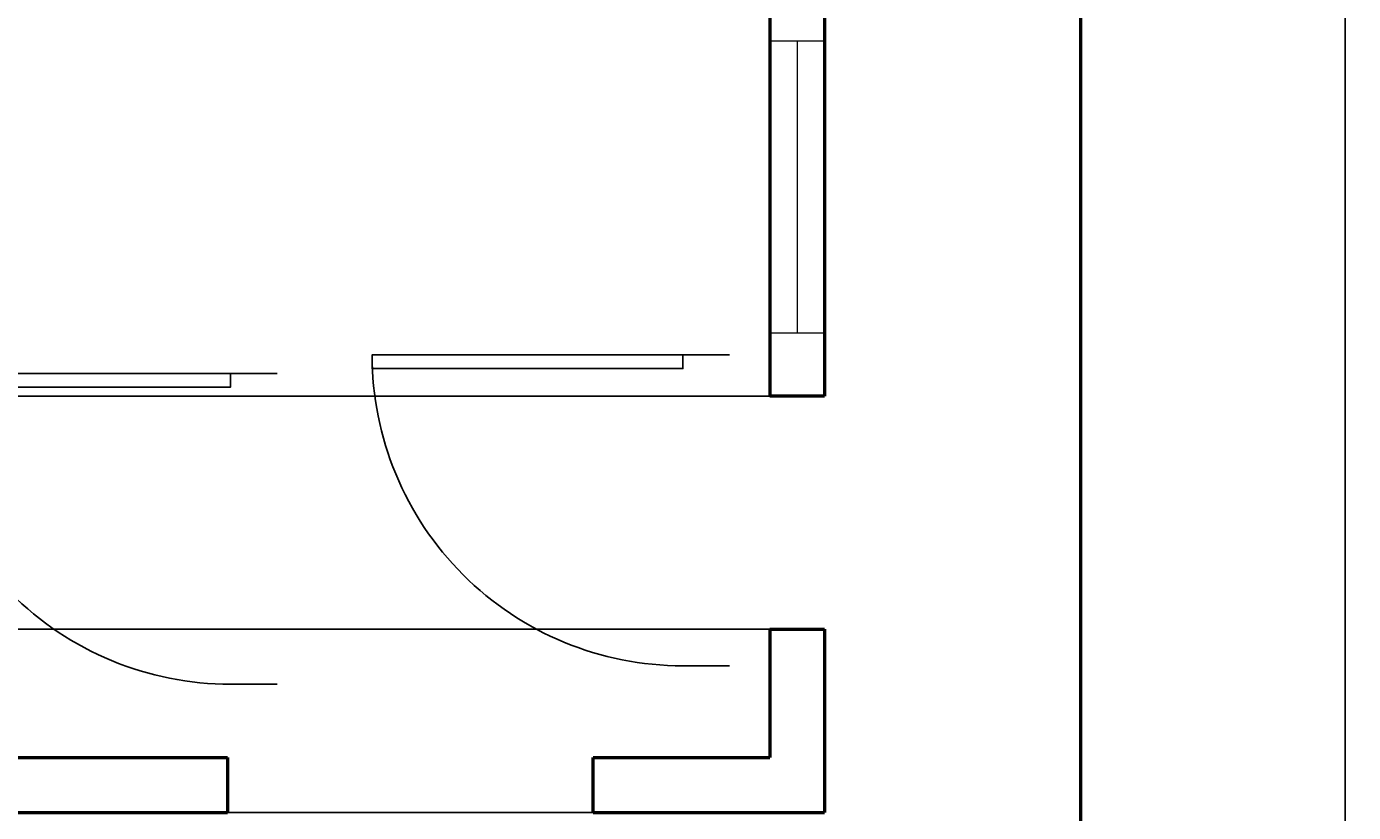
# Model space of a CAD drawing. Units: inches. Extents: x 3506 to 3958, y 1553 to 2506.
# Tile 7 of 16: x 3739 to 3957, y 1770 to 1899. Entities that reach past the tile are written whole.
import ezdxf

# ---------------------------------------------------------------- set-up
doc = ezdxf.new("R2010")
doc.units = ezdxf.units.IN
doc.header["$MEASUREMENT"] = 0
for name, color, linetype, lineweight in [('A-ANNO-DIMS', 2, 'Continuous', 18), ('A-FLOR-STRS', 7, 'Continuous', 25), ('A-WALL', 7, 'Continuous', 50), ('doors', 40, 'Continuous', 25), ('window', 30, 'Continuous', 20)]:
    doc.layers.add(name, color=color, linetype=linetype, lineweight=lineweight)
doc.layers.add('A-WALL-PATT', color=251, linetype='Continuous', lineweight=13, true_color=0x636466)
doc.styles.get("Standard").update_dxf_attribs({"font": 'arial.ttf'})
doc.dimstyles.get("Standard").update_dxf_attribs({"dimtxt": 1.18, "dimasz": 0.68, "dimexe": 0.18, "dimexo": 0.0625, "dimgap": 0.09, "dimtad": 0, "dimtih": 1, "dimtoh": 1, "dimdec": 1, "dimzin": 0, "dimdsep": 46, "dimlunit": 3, "dimtxsty": 'Standard', "dimcen": 0.09, "dimadec": 0, "dimazin": 0, "dimtfac": 1, "dimtdec": 1, "dimtofl": 0, "dimtmove": 0, "dimatfit": 3, "dimfxl": 1, "dimtolj": 1, "dimtzin": 0, "dimarcsym": 0})

# ---------------------------------------------------------------- blocks, each defined once
blk = doc.blocks.new('*U12')
for p, q in [((0, 0), (0, 6)), ((40, 0), (40, 6))]:
    blk.add_line(p, q)
blk.add_lwpolyline([(0, 0), (0, -40), (1.75, -40), (1.75, 0)], close=True)
blk.add_arc((0, 0), 40, 270, 0)
blk = doc.blocks.new('*D39')
at = {"layer": 'A-ANNO-DIMS', "color": 0, "lineweight": -2, "transparency": 16777216}
for p, q in [((3911.79, 2461.39), (3955.36, 2461.39)), ((3955.18, 2460.71), (3955.18, 2030.09)), ((3955.18, 1598.07), (3955.18, 2028.7)), ((3911.79, 1597.39), (3955.36, 1597.39))]:
    blk.add_line(p, q, dxfattribs=at)
at = {"layer": 'A-ANNO-DIMS', "color": 0, "transparency": 16777216}
for points in [[(3955.07, 2460.71), (3955.29, 2460.71), (3955.18, 2461.39)], [(3955.07, 1598.07), (3955.29, 1598.07), (3955.18, 1597.39)]]:
    blk.add_solid(points, dxfattribs=at)
at = {"layer": 'Defpoints', "color": 0, "transparency": 16777216}
for p in [(3911.73, 2461.39), (3955.18, 2461.39), (3911.73, 1597.39)]:
    blk.add_point(p, dxfattribs=at)
at = {"layer": 'A-ANNO-DIMS', "color": 0, "transparency": 16777216, "insert": (3955.18, 2029.39), "char_height": 1.18, "attachment_point": 5}
blk.add_mtext('\\A1;864', dxfattribs=at)
blk = doc.blocks.new('*D62')
at = {"layer": 'A-ANNO-DIMS', "color": 0, "lineweight": -2, "transparency": 16777216}
for p, q in [((3860.67, 1838.71), (3508.1, 1838.71)), ((3508.28, 1838.03), (3508.28, 1820.28)), ((3508.28, 1801.14), (3508.28, 1818.89)), ((3860.67, 1800.46), (3508.1, 1800.46))]:
    blk.add_line(p, q, dxfattribs=at)
at = {"layer": 'A-ANNO-DIMS', "color": 0, "transparency": 16777216}
for points in [[(3508.17, 1838.03), (3508.39, 1838.03), (3508.28, 1838.71)], [(3508.17, 1801.14), (3508.39, 1801.14), (3508.28, 1800.46)]]:
    blk.add_solid(points, dxfattribs=at)
at = {"layer": 'Defpoints', "color": 0, "transparency": 16777216}
for p in [(3860.73, 1838.71), (3508.28, 1800.46), (3860.73, 1800.46)]:
    blk.add_point(p, dxfattribs=at)
at = {"layer": 'A-ANNO-DIMS', "color": 0, "transparency": 16777216, "insert": (3508.28, 1819.59), "char_height": 1.18, "attachment_point": 5}
blk.add_mtext('\\A1;38.246', dxfattribs=at)
blk = doc.blocks.new('*D63')
at = {"layer": 'A-ANNO-DIMS', "color": 0, "lineweight": -2, "transparency": 16777216}
for p, q in [((3869.67, 1800.46), (3508.1, 1800.46)), ((3508.28, 1799.78), (3508.28, 1786.12)), ((3508.28, 1771.07), (3508.28, 1784.74)), ((3869.67, 1770.39), (3508.1, 1770.39))]:
    blk.add_line(p, q, dxfattribs=at)
at = {"layer": 'A-ANNO-DIMS', "color": 0, "transparency": 16777216}
for points in [[(3508.17, 1799.78), (3508.39, 1799.78), (3508.28, 1800.46)], [(3508.17, 1771.07), (3508.39, 1771.07), (3508.28, 1770.39)]]:
    blk.add_solid(points, dxfattribs=at)
at = {"layer": 'Defpoints', "color": 0, "transparency": 16777216}
for p in [(3869.73, 1800.46), (3508.28, 1770.39), (3869.73, 1770.39)]:
    blk.add_point(p, dxfattribs=at)
at = {"layer": 'A-ANNO-DIMS', "color": 0, "transparency": 16777216, "insert": (3508.28, 1785.43), "char_height": 1.18, "attachment_point": 5}
blk.add_mtext('\\A1;30.07', dxfattribs=at)

msp = doc.modelspace()

# ---------------------------------------------------------------- hatches: boundary and pattern name
at = {"layer": 'A-WALL-PATT'}
h = msp.add_hatch(dxfattribs=at)
h.set_pattern_fill('ANSI31', color=256)
h.paths.add_polyline_path([(3911.7302, 2461.3942), (3551.7302, 2461.3942), (3551.7302, 2152.516), (3560.7302, 2152.516), (3560.7302, 2116.516), (3551.7302, 2116.516), (3551.7302, 1920.5711), (3556.2302, 1920.5711), (3560.7302, 1920.5711), (3560.7302, 2000.3942), (3692.7302, 2000.3942), (3692.7302, 1997.3942), (3697.7302, 1997.3942), (3697.7302, 2000.3942), (3771.7302, 2000.3942), (3771.7302, 1997.3942), (3776.7302, 1997.3942), (3776.7302, 1997.7206), (3778.5802, 1997.7206), (3807.5802, 1997.7206), (3807.5802, 1996.4519), (3778.5802, 1996.4519), (3778.5802, 1997.7206), (3776.7302, 1997.7206), (3776.7302, 1997.3942), (3771.7302, 1997.3942), (3771.7302, 2000.3942), (3697.7302, 2000.3942), (3697.7302, 1997.3942), (3692.7302, 1997.3942), (3689.8302, 1997.3942), (3689.8302, 1995.8192), (3653.8302, 1995.8192), (3653.8302, 1997.3942), (3689.8302, 1997.3942), (3692.7302, 1997.3942), (3692.7302, 2000.3942), (3560.7302, 2000.3942), (3560.7302, 1920.5711), (3551.7302, 1920.5711), (3551.7302, 1884.5711), (3551.7302, 1597.3942), (3911.7302, 1597.3942)], flags=17)
h.paths.add_polyline_path([(3596.7302, 2005.3942), (3596.7302, 2057.3035, -0.38730371), (3569.1778, 2085), (3569.15, 2085), (3569.15, 2086.2688), (3598.15, 2086.2688), (3598.15, 2085), (3569.1778, 2085, 0.38730371), (3596.7302, 2057.3035), (3596.7302, 2057.3942), (3601.7302, 2057.3942), (3601.7302, 2055.3942), (3630.7302, 2055.3942), (3630.7302, 2034.3942), (3694.7302, 2034.3942), (3694.7302, 2053.3942), (3699.7302, 2053.3942), (3699.7302, 2005.3942), (3860.7302, 2005.3942), (3860.7302, 2173.3942), (3771.7302, 2173.3942), (3771.7302, 2194.3942), (3776.7302, 2194.3942), (3776.7302, 2178.3942), (3860.7302, 2178.3942), (3860.7302, 2231.3942), (3601.7302, 2231.3942), (3601.7302, 2241.426), (3596.7302, 2241.426), (3596.7302, 2231.3942), (3560.7302, 2231.3942), (3560.7302, 2315.3942), (3596.7302, 2315.3942), (3596.7302, 2312.3942), (3601.7302, 2312.3942), (3601.7302, 2315.3942), (3697.7302, 2315.3942), (3697.7302, 2413.3942), (3692.7302, 2413.3942), (3692.7302, 2320.3942), (3560.7302, 2320.3942), (3560.7302, 2452.3942), (3692.7302, 2452.3942), (3692.7302, 2449.3942), (3697.7302, 2449.3942), (3697.7302, 2452.3942), (3771.7302, 2452.3942), (3771.7302, 2449.3942), (3776.7302, 2449.3942), (3776.7302, 2452.3942), (3860.7302, 2452.3942), (3860.7302, 2437.2075), (3865.2302, 2437.2075), (3865.2302, 2413.2075), (3860.7302, 2413.2075), (3860.7302, 2367.6976), (3865.2302, 2367.6976), (3869.7302, 2367.6976), (3869.7302, 2319.6976), (3860.7302, 2319.6976), (3860.7302, 2211.6248), (3869.7302, 2211.6248), (3869.7302, 2187.6248), (3860.7302, 2187.6248), (3860.7302, 2138.4346), (3865.2302, 2138.4346), (3869.7302, 2138.4346), (3869.7302, 2090.4346), (3860.7302, 2090.4346), (3860.7302, 1985.8449), (3869.7302, 1985.8449), (3869.7302, 1961.8449), (3860.7302, 1961.8449), (3860.7302, 1897.0756), (3865.2302, 1897.0756), (3869.7302, 1897.0756), (3869.7302, 1849.0756), (3860.7302, 1849.0756), (3860.7302, 1847.8112), (3860.7302, 1779.3942), (3596.7302, 1779.3942), (3596.7302, 1831.3942), (3601.7302, 1831.3942), (3601.7302, 1828.3942), (3630.7302, 1828.3942), (3630.7302, 1808.3942), (3691.7302, 1808.3942), (3691.7302, 1815.3942), (3696.7302, 1815.3942), (3696.7302, 1779.3942), (3860.7302, 1779.3942), (3860.7302, 1947.3942), (3771.7302, 1947.3942), (3771.7302, 1968.3942), (3776.7302, 1968.3942), (3776.7302, 1952.3942), (3860.7302, 1952.3942), (3860.7302, 2005.3942)], flags=0)
h.paths.add_polyline_path([(3596.7302, 2038.8546), (3601.7302, 2038.8546), (3601.7302, 2014.8546), (3596.7302, 2014.8546)], flags=0)
h.paths.add_polyline_path([(3564.1688, 2107), (3564.1688, 2167), (3644.1688, 2167), (3644.1688, 2107)], flags=0)
h.paths.add_polyline_path([(3607.0972, 2052.0208), (3620.8472, 2052.0208, -0.41421356), (3621.9931, 2050.875), (3621.9931, 2025.6667, -0.41421356), (3620.8472, 2024.5208), (3607.0972, 2024.5208, -0.41421356), (3605.9514, 2025.6667), (3605.9514, 2050.875, -0.41421356)], flags=0)
h.paths.add_polyline_path([(3578.5688, 2115), (3565.3688, 2115), (3565.3688, 2135.8), (3578.5688, 2135.8), (3578.5688, 2138.2), (3565.3688, 2138.2), (3565.3688, 2159), (3580.5688, 2159), (3580.5688, 2153.8), (3593.7688, 2167), (3593.7688, 2151.8), (3578.5688, 2151.8)], flags=0)
h.paths.add_polyline_path([(3610.9167, 2050.875), (3620.0833, 2050.875, -0.41421356), (3620.8472, 2050.1111), (3620.8472, 2039.6076, -0.41421356), (3620.0833, 2038.8438), (3610.9167, 2038.8438, -0.41421356), (3610.1528, 2039.6076), (3610.1528, 2050.1111, -0.41421356)], flags=0)
h.paths.add_polyline_path([(3610.9167, 2037.6979), (3620.0833, 2037.6979, -0.41421356), (3620.8472, 2036.934), (3620.8472, 2026.4306, -0.41421356), (3620.0833, 2025.6667), (3610.9167, 2025.6667, -0.41421356), (3610.1528, 2026.4306), (3610.1528, 2036.934, -0.41421356)], flags=0)
h.paths.add_polyline_path([(3616.2639, 2044.7639, -1), (3614.7361, 2044.7639, -1)], flags=0)
h.paths.add_polyline_path([(3615.8819, 2044.7639, -1), (3615.1181, 2044.7639, -1)], flags=0)
h.paths.add_polyline_path([(3616.2639, 2031.7778, -1), (3614.7361, 2031.7778, -1)], flags=0)
h.paths.add_polyline_path([(3615.8819, 2031.7778, -1), (3615.1181, 2031.7778, -1)], flags=0)
h.paths.add_polyline_path([(3609.7539, 2021.7868), (3626.9586, 2021.7868), (3626.9586, 2008.8833), (3609.7539, 2008.8833)], flags=0)
h.paths.add_polyline_path([(3610.4708, 2021.07), (3621.2237, 2021.07), (3621.2237, 2009.6002), (3610.4708, 2009.6002)], flags=0)
h.paths.add_polyline_path([(3611.5461, 2019.9947), (3620.1484, 2019.9947), (3620.1484, 2010.6755), (3611.5461, 2010.6755)], flags=0)
h.paths.add_polyline_path([(3621.9405, 2021.07), (3626.2417, 2021.07), (3626.2417, 2009.6002), (3621.9405, 2009.6002)], flags=0)
h.paths.add_polyline_path([(3622.6574, 2020.3531), (3625.5248, 2020.3531), (3625.5248, 2017.4857), (3622.6574, 2017.4857)], flags=0)
h.paths.add_polyline_path([(3622.6574, 2016.7688), (3625.5248, 2016.7688), (3625.5248, 2010.317), (3622.6574, 2010.317)], flags=0)
h.paths.add_polyline_path([(3624.808, 2016.0519), (3624.808, 2013.9013), (3624.0911, 2013.9013), (3624.0911, 2013.1845), (3623.3743, 2013.1845), (3623.3743, 2013.9013), (3623.3743, 2016.0519)], flags=0)
h.paths.add_polyline_path([(3623.0158, 2012.8261), (3625.1664, 2012.8261), (3625.1664, 2012.1092), (3623.0158, 2012.1092)], flags=0)
h.paths.add_polyline_path([(3623.0158, 2011.7508), (3625.1664, 2011.7508), (3625.1664, 2011.0339), (3623.0158, 2011.0339)], flags=0)
h.paths.add_polyline_path([(3650.0591, 2031.8202), (3674.0368, 2031.8202), (3674.0368, 2012.638), (3669.2413, 2012.638), (3669.2413, 2011.8388), (3672.4383, 2011.8388), (3672.4383, 2011.0395), (3651.6576, 2011.0395), (3651.6576, 2011.8388), (3654.8546, 2011.8388), (3654.8546, 2012.638), (3650.0591, 2012.638)], flags=0)
h.paths.add_polyline_path([(3658.0517, 2024.6269, -1), (3651.6576, 2024.6269, -1)], flags=0)
h.paths.add_polyline_path([(3657.2524, 2024.6269, -1), (3652.4569, 2024.6269, -1)], flags=0)
h.paths.add_polyline_path([(3656.4532, 2024.6269, -1), (3653.2561, 2024.6269, -1)], flags=0)
h.paths.add_polyline_path([(3655.6539, 2024.6269, -1), (3654.0554, 2024.6269, -1)], flags=0)
h.paths.add_polyline_path([(3657.2524, 2017.4336, -1), (3652.4569, 2017.4336, -1)], flags=0)
h.paths.add_polyline_path([(3656.4532, 2017.4336, -1), (3653.2561, 2017.4336, -1)], flags=0)
h.paths.add_polyline_path([(3655.6539, 2017.4336, -1), (3654.0554, 2017.4336, -1)], flags=0)
h.paths.add_polyline_path([(3659.6502, 2027.8239), (3664.4457, 2027.8239), (3664.4457, 2015.0358), (3659.6502, 2015.0358)], flags=0)
h.paths.add_polyline_path([(3663.6465, 2027.0247), (3663.6465, 2015.8351), (3660.4494, 2015.8351), (3660.4494, 2027.0247)], flags=0)
h.paths.add_polyline_path([(3562.6688, 1945.5), (3642.6688, 1945.5), (3642.6688, 1885.5), (3562.6688, 1885.5)], flags=0)
h.paths.add_polyline_path([(3671.6391, 2024.6269, -1), (3666.8435, 2024.6269, -1)], flags=0)
h.paths.add_polyline_path([(3670.8398, 2024.6269, -1), (3667.6428, 2024.6269, -1)], flags=0)
h.paths.add_polyline_path([(3672.4383, 2017.4336, -1), (3666.0443, 2017.4336, -1)], flags=0)
h.paths.add_polyline_path([(3670.0405, 2024.6269, -1), (3668.442, 2024.6269, -1)], flags=0)
h.paths.add_polyline_path([(3671.6391, 2017.4336, -1), (3666.8435, 2017.4336, -1)], flags=0)
h.paths.add_polyline_path([(3670.8398, 2017.4336, -1), (3667.6428, 2017.4336, -1)], flags=0)
h.paths.add_polyline_path([(3592.2688, 1945.5), (3592.2688, 1930.3), (3577.0688, 1930.3), (3577.0688, 1893.5), (3563.8688, 1893.5), (3563.8688, 1914.3), (3577.0688, 1914.3), (3577.0688, 1916.7), (3563.8688, 1916.7), (3563.8688, 1937.5), (3579.0688, 1937.5), (3579.0688, 1932.3)], flags=0)
h.paths.add_polyline_path([(3670.0405, 2017.4336, -1), (3668.442, 2017.4336, -1)], flags=0)
h.paths.add_polyline_path([(3596.7302, 2283.3942), (3601.7302, 2283.3942), (3601.7302, 2265.426), (3599.2302, 2265.426), (3599.2302, 2241.426), (3596.7302, 2241.426), (3596.7302, 2265.426)], flags=0)
h.paths.add_polyline_path([(3596.7302, 1810.7006), (3601.7302, 1810.7006), (3601.7302, 1786.7006), (3596.7302, 1786.7006)], flags=0)
h.paths.add_polyline_path([(3560.7302, 1770.3942), (3738.7302, 1770.3942), (3738.7302, 1746.3942), (3738.7302, 1722.3942), (3748.7302, 1722.3942), (3748.7302, 1674.3942), (3560.7302, 1674.3942)], flags=0)
h.paths.add_polyline_path([(3728.7302, 1746.3942), (3728.7302, 1756.0642), (3738.7302, 1746.3942), (3728.7302, 1738.1582), (3728.7302, 1698.3942), (3591.2519, 1698.3942), (3591.2519, 1746.3942)], flags=0)
h.paths.add_polyline_path([(3771.7302, 2399.3942), (3771.7302, 2420.3942), (3776.7302, 2420.3942), (3776.7302, 2404.3942), (3776.7302, 2399.3942)], flags=0)
h.paths.add_polyline_path([(3911.7302, 2461.3942), (3551.7302, 2461.3942), (3551.7302, 2152.516), (3560.7302, 2152.516), (3560.7302, 2116.516), (3551.7302, 2116.516), (3551.7302, 1920.5711), (3560.7302, 1920.5711), (3560.7302, 2000.3942), (3692.7302, 2000.3942), (3692.7302, 1997.3942), (3697.7302, 1997.3942), (3697.7302, 2000.3942), (3771.7302, 2000.3942), (3771.7302, 1997.3942), (3776.7302, 1997.3942), (3776.7302, 1997.7206), (3778.5802, 1997.7206), (3807.5802, 1997.7206), (3807.5802, 1996.4519), (3778.5802, 1996.4519), (3778.5802, 1997.7206), (3776.7302, 1997.7206), (3776.7302, 1997.3942), (3771.7302, 1997.3942), (3771.7302, 2000.3942), (3697.7302, 2000.3942), (3697.7302, 1997.3942), (3692.7302, 1997.3942), (3689.8302, 1997.3942), (3689.8302, 1995.8192), (3653.8302, 1995.8192), (3653.8302, 1997.3942), (3689.8302, 1997.3942), (3692.7302, 1997.3942), (3692.7302, 2000.3942), (3560.7302, 2000.3942), (3560.7302, 1920.5711), (3551.7302, 1920.5711), (3551.7302, 1597.3942), (3911.7302, 1597.3942)], flags=17)

# ---------------------------------------------------------------- linework, layer by layer
at = {"layer": 'A-FLOR-STRS'}
msp.add_line((3608.7302, 1770.3942), (3771.7302, 1770.3942), dxfattribs=at)
at = {"layer": 'A-WALL'}
for p, q in [((3860.7302, 2015.4906), (3860.7302, 1838.7087)), ((3869.7302, 2015.4906), (3869.7302, 1838.7087)), ((3869.7302, 1838.7087), (3860.7302, 1838.7087)), ((3860.7302, 1800.4628), (3869.7302, 1800.4628)), ((3860.7302, 1800.4628), (3860.7302, 1779.3942)), ((3869.7302, 1800.4628), (3869.7302, 1770.3942)), ((3560.7302, 1779.3942), (3771.7302, 1779.3942)), ((3771.7302, 1779.3942), (3771.7302, 1770.3942)), ((3831.7302, 1779.3942), (3860.7302, 1779.3942)), ((3831.7302, 1770.3942), (3831.7302, 1779.3942)), ((3831.7302, 1779.3942), (3860.7302, 1779.3942)), ((3560.7302, 1770.3942), (3771.7302, 1770.3942)), ((3831.7302, 1770.3942), (3860.7302, 1770.3942)), ((3831.7302, 1770.3942), (3869.7302, 1770.3942))]:
    msp.add_line(p, q, dxfattribs=at)
msp.add_lwpolyline([(3551.7302, 2461.3942), (3911.7302, 2461.3942), (3911.7302, 1597.3942), (3551.7302, 1597.3942)], close=True, dxfattribs=at)
at = {"layer": 'window'}
for p, q in [((3860.7302, 1897.0756), (3869.7302, 1897.0756)), ((3860.7302, 1897.0756), (3865.2302, 1897.0756)), ((3865.2302, 1897.0756), (3865.2302, 1849.0756)), ((3869.7302, 1897.0756), (3869.7302, 1849.0756)), ((3860.7302, 1895.8112), (3860.7302, 1847.8112)), ((3869.7302, 1849.0756), (3860.7302, 1849.0756))]:
    msp.add_line(p, q, dxfattribs=at)

# ---------------------------------------------------------------- block references
at = {"layer": 'doors', "xscale": 1.27563568336709, "yscale": 1.27563568336709, "zscale": 1.27563568336709, "rotation": 270}
for p in [(3846.4757, 1845.4859), (3772.2282, 1842.4626)]:
    msp.add_blockref('*U12', p, dxfattribs=at)

# ---------------------------------------------------------------- dimensions: what is measured, and where the dimension line sits
at = {"layer": 'A-ANNO-DIMS'}
for base, p1, p2, override, picture, middle in [((3955.1802, 2461.3942), (3911.7302, 1597.3942), (3911.7302, 2461.3942), {"dimdec": 0, "dimlfac": 1, "dimrnd": 0, "dimzin": 0, "dimdsep": 46, "dimlunit": 2}, '*D39', (3955.1802, 2029.3942)), ((3508.2802, 1800.4628), (3860.7302, 1838.7087), (3860.7302, 1800.4628), {"dimdec": 3, "dimlfac": 1, "dimrnd": 0, "dimzin": 0, "dimdsep": 46, "dimlunit": 2}, '*D62', (3508.2802, 1819.5857)), ((3508.2802, 1770.3942), (3869.7302, 1800.4628), (3869.7302, 1770.3942), {"dimdec": 2, "dimlfac": 1, "dimrnd": 0, "dimzin": 0, "dimdsep": 46, "dimlunit": 2}, '*D63', (3508.2802, 1785.4285))]:
    dim = msp.add_linear_dim(base=base, p1=p1, p2=p2, angle=90, dimstyle='Standard', override=override, dxfattribs=at)
    dim.commit()
    dim.dimension.update_dxf_attribs({"geometry": picture, "text_midpoint": middle})

doc.saveas('drawing.dxf')
